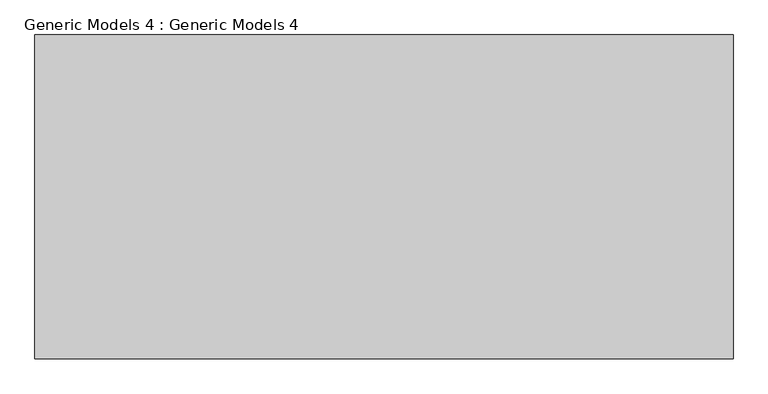
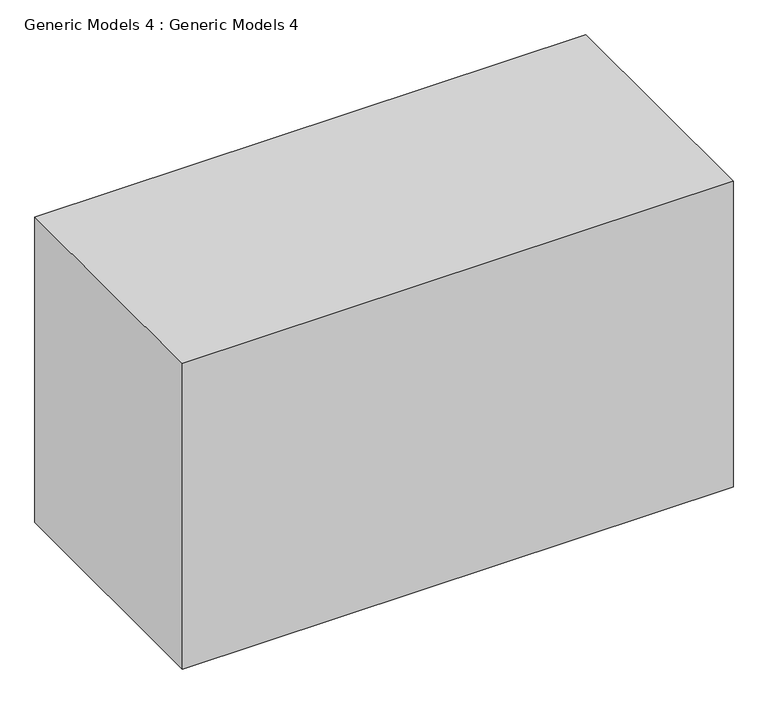
"""IFC4 building model written with IfcOpenShell, lengths in millimetres: proxy geometry, Generic Models 4 : Generic Models 4."""

from ifc_helpers import new_model, si_unit, frame, origin, place, context, project, spatial, polyline, outline, extrude, source, transform, mapped, element, save


def generic_models_4_generic_models_4_92c2c5ab(model_context):
    return source(origin(), model_context, "Body", "SweptSolid", [
        extrude(outline(polyline([(-6274.229521, -14340.8001929), (-12103.529521, -14340.8001929), (-12103.529521, -11635.7001929), (-6274.229521, -11635.7001929), (-6274.229521, -14340.8001929)])), frame((0.0, 0.0, 6400.8), z_axis=(0.0, 0.0, 1.0), x_axis=(1.0, 0.0, 0.0)), (0.0, 0.0, 1.0), 3421.8068762),
    ])


if __name__ == "__main__":
    model = new_model("IFC4")
    model_context = context("Model", 3, world=origin())
    ifc_project = project(units=[si_unit("LENGTHUNIT", "METRE", prefix="MILLI")], contexts=[model_context])
    site = spatial("IfcSite", under=ifc_project)
    building = spatial("IfcBuilding", under=site)
    placement = place(None, origin())
    generic_models_4_generic_models_4_shape = generic_models_4_generic_models_4_92c2c5ab(model_context)
    element("IfcBuildingElementProxy", 1, Name="Generic Models 4 : Generic Models 4", ObjectType="Generic Models 4 : Generic Models 4", at=placement, inside=building, context=model_context, shape_type="MappedRepresentation", body=[
        mapped(generic_models_4_generic_models_4_shape, transform((0.0, 0.0, 0.0), x_axis=(1.0, 0.0, 0.0), y_axis=(0.0, 1.0, 0.0), z_axis=(0.0, 0.0, 1.0))),
    ])
    save(model, "model.ifc")
